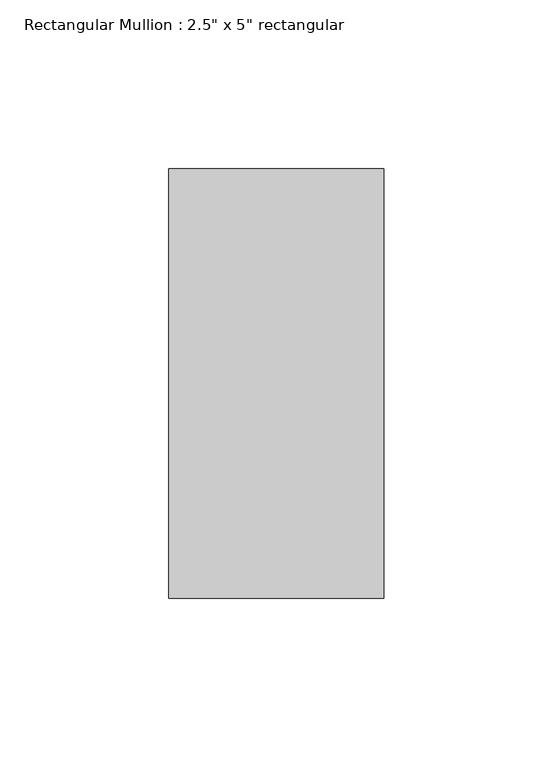
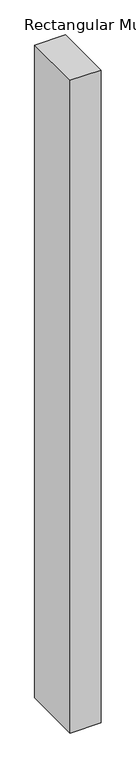
"""IFC4 building model written with IfcOpenShell, lengths in millimetres: member geometry."""

from ifc_helpers import new_model, si_unit, frame, origin, place, context, project, spatial, polyline, outline, extrude, source, transform, mapped, element, save


def member_80b92b34(model_context):
    return source(origin(), model_context, "Body", "SweptSolid", [
        extrude(outline(polyline([(0.0, 63.5), (0.0, -63.5), (-63.5, -63.5), (-63.5, 63.5), (0.0, 63.5)])), frame((0.0, 0.0, -1422.1292854), z_axis=(0.0, 0.0, 1.0), x_axis=(1.0, 0.0, 0.0)), (0.0, 0.0, 1.0), 1422.1292854),
    ])


if __name__ == "__main__":
    model = new_model("IFC4")
    model_context = context("Model", 3, world=origin())
    ifc_project = project(units=[si_unit("LENGTHUNIT", "METRE", prefix="MILLI")], contexts=[model_context])
    site = spatial("IfcSite", under=ifc_project)
    building = spatial("IfcBuilding", under=site)
    placement = place(None, origin())
    member_shape = member_80b92b34(model_context)
    element("IfcMember", 1, ObjectType="Rectangular Mullion : 2.5\" x 5\" rectangular", at=placement, inside=building, context=model_context, shape_type="MappedRepresentation", body=[
        mapped(member_shape, transform((0.0, 0.0, 0.0), x_axis=(1.0, 0.0, 0.0), y_axis=(0.0, 1.0, 0.0), z_axis=(0.0, 0.0, 1.0))),
    ])
    save(model, "model.ifc")

# Revit data of these elements
# Type "Rectangular Mullion : 2.5\" x 5\" rectangular"
#   built-in parameter 1007304 = 0.416667 (stored number, unit not read)
#   built-in parameter 1007301 = 0.104167 (stored number, unit not read)
#   built-in parameter 1007300 = 0.104167 (stored number, unit not read)
# Element 1 (IfcMember, "Rectangular Mullion : 2.5\" x 5\" rectangular")
#   Materials on its faces: "Aluminum"
# Materials
#   "Aluminum": class "Metal", colour RGB 247 247 247, transparency 0, Description = "Aluminum 6061", Cost = 0
